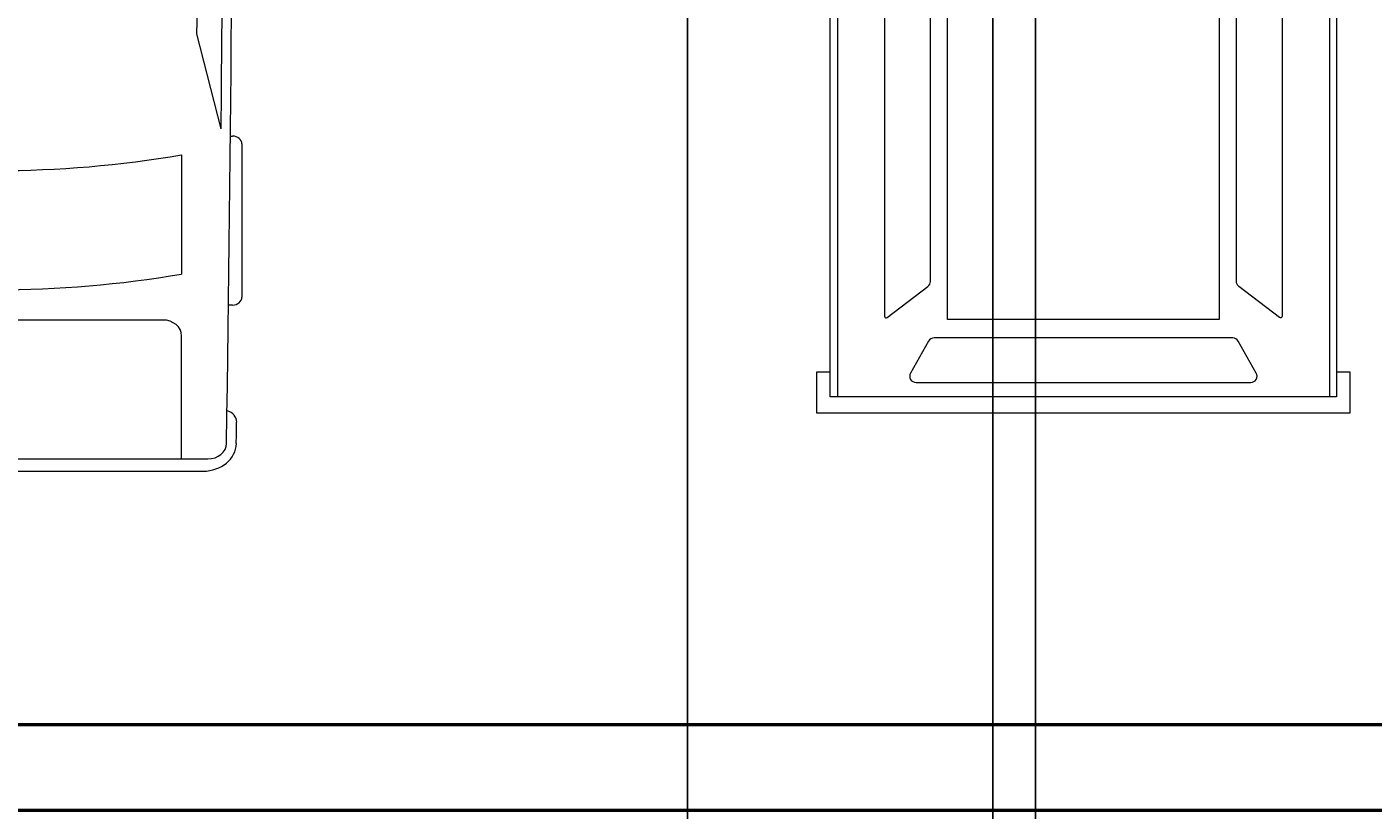
# Model space of a CAD drawing. Units: inches. Extents: x 5375 to 6084, y 16106 to 17259.
# Tile 10 of 32: x 5844 to 5986, y 16212 to 16295. Entities that reach past the tile are written whole.
import ezdxf

# ---------------------------------------------------------------- set-up
doc = ezdxf.new("R2010")
doc.units = ezdxf.units.IN
for name, color, linetype, lineweight in [('A-ANNO-DIMS', 2, 'Continuous', 18), ('C-PKNG-VEHI', 7, 'Continuous', 13), ('WALL', 6, 'Continuous', 50)]:
    doc.layers.add(name, color=color, linetype=linetype, lineweight=lineweight)
doc.styles.get("Standard").update_dxf_attribs({"font": 'arial.ttf'})
doc.dimstyles.get("Standard").update_dxf_attribs({"dimtxt": 0.18, "dimasz": 0.18, "dimexe": 0.18, "dimexo": 0.0625, "dimgap": 0.09, "dimtad": 0, "dimtih": 1, "dimtoh": 1, "dimdec": 4, "dimzin": 0, "dimdsep": 46, "dimtxsty": 'Standard', "dimcen": 0.09, "dimadec": 0, "dimazin": 0, "dimtfac": 1, "dimtdec": 4, "dimtofl": 0, "dimtmove": 0, "dimatfit": 3, "dimfxl": 1, "dimtolj": 1, "dimtzin": 0, "dimarcsym": 0})

# ---------------------------------------------------------------- blocks, each defined once
blk = doc.blocks.new('*U9')
for p, q in [((136.7, 38.89), (160.9, 38.89)), ((135.45, 37.07), (135.45, 37.41)), ((162.15, 37.41), (162.15, 36.77)), ((134.31, 35.6), (119.29, 31.78)), ((186.47, -33.5), (186.47, 33.5)), ((188.4, -32.76), (188.4, 32.76)), ((138.42, 29.35), (157.25, 29.35)), ((186.47, 29.35), (167.01, 29.35)), ((164.52, 26.39), (164.52, -26.39)), ((186.47, -10.53), (186.47, 10.53))]:
    blk.add_line(p, q)
for centre, major_axis, start_param, end_param in [((136.7, 37.41), (0, -1.48), 3.141593, 4.712389), ((160.9, 37.41), (0, 1.48), -1.570796, 0), ((64.48, -10555.62), (0, 10593.03), -0.013397, 0.002797), ((180.63, 35.84), (0, 2.22), -0.013017, 1.249894), ((64.48, -10556.36), (0, 10595.31), -0.013397, -0.013017), ((183.98, 33.5), (0, -2.96), 1.570796, 3.128196), ((183.98, 32.76), (0, -5.25), 1.570796, 3.128196), ((64.48, -10555.62), (0, -10591.55), 3.133765, 3.140441), ((95.79, -3666.35), (0, -3698.24), 3.134049, 3.144098), ((17.08, 0), (0, 147.02), 4.511394, 4.913384), ((35.91, 0), (0, 147.02), 4.511394, 4.913384), ((167.01, 26.39), (0, 2.96), 0, 1.570796)]:
    blk.add_ellipse(centre, major_axis=major_axis, ratio=0.842304, start_param=start_param, end_param=end_param)
blk = doc.blocks.new('*U10')
for p, q in [((1.28, 38.87), (175.66, 38.87)), ((1.28, -38.87), (175.66, -38.87))]:
    blk.add_line(p, q)
for points in [[(171.74, 40.01), (175.66, 40.01), (175.66, -40.01), (171.74, -40.01), (171.74, -42.18), (178.14, -42.18), (178.14, 42.18), (171.74, 42.18)], [(1.28, 40.01), (175.66, 40.01), (175.66, -40.01), (1.28, -40.01)], [(71.47, 21.48), (163.42, 21.48), (163.42, -21.48), (71.47, -21.48)]]:
    blk.add_lwpolyline(points, close=True)
for points in [[(102.19, 24.58), (106.97, 31, -0.236929), (107.78, 31.41), (162.91, 31.41, -0.621576), (163.11, 31), (158.19, 24.58, -0.233368), (157.39, 24.18), (102.39, 24.18, -0.616908)], [(171.88, 27.31), (166.83, 24.47, 0.271143), (166.32, 23.6), (166.32, -23.6, 0.271143), (166.83, -24.47), (171.88, -27.31, 0.573387), (173.37, -26.44), (173.37, 26.44, 0.573387)], [(102.19, -24.58), (106.97, -31, 0.236929), (107.78, -31.41), (162.91, -31.41, 0.621576), (163.11, -31), (158.19, -24.58, 0.233368), (157.39, -24.18), (102.39, -24.18, 0.616908)]]:
    blk.add_lwpolyline(points, format="xyb", close=True)
blk = doc.blocks.new('*D44')
at = {"layer": 'A-ANNO-DIMS', "color": 0, "lineweight": -2, "transparency": 16777216}
for p, q in [((5914, 16886.53), (5914, 16106.48)), ((5946.12, 16886.53), (5946.12, 16106.48)), ((5914.18, 16106.66), (5929.6, 16106.66)), ((5945.94, 16106.66), (5930.53, 16106.66))]:
    blk.add_line(p, q, dxfattribs=at)
at = {"layer": 'A-ANNO-DIMS', "color": 0, "transparency": 16777216}
for points in [[(5914.18, 16106.69), (5914.18, 16106.63), (5914, 16106.66)], [(5945.94, 16106.69), (5945.94, 16106.63), (5946.12, 16106.66)]]:
    blk.add_solid(points, dxfattribs=at)
at = {"layer": 'Defpoints', "color": 0, "transparency": 16777216}
for p in [(5914, 16886.6), (5946.12, 16886.6), (5914, 16106.66)]:
    blk.add_point(p, dxfattribs=at)
at = {"layer": 'A-ANNO-DIMS', "color": 0, "transparency": 16777216, "insert": (5930.06, 16106.66), "char_height": 0.18, "attachment_point": 5}
blk.add_mtext('\\A1;32.117', dxfattribs=at)
blk = doc.blocks.new('*D46')
at = {"layer": 'A-ANNO-DIMS', "color": 0, "lineweight": -2, "transparency": 16777216}
for p, q in [((5946.12, 16771.52), (5946.12, 16106.48)), ((5950.62, 16771.52), (5950.62, 16106.48)), ((5946.3, 16106.66), (5948.11, 16106.66)), ((5950.44, 16106.66), (5948.63, 16106.66))]:
    blk.add_line(p, q, dxfattribs=at)
at = {"layer": 'A-ANNO-DIMS', "color": 0, "transparency": 16777216}
for points in [[(5946.3, 16106.69), (5946.3, 16106.63), (5946.12, 16106.66)], [(5950.44, 16106.69), (5950.44, 16106.63), (5950.62, 16106.66)]]:
    blk.add_solid(points, dxfattribs=at)
at = {"layer": 'Defpoints', "color": 0, "transparency": 16777216}
for p in [(5946.12, 16771.58), (5950.62, 16771.58), (5950.62, 16106.66)]:
    blk.add_point(p, dxfattribs=at)
at = {"layer": 'A-ANNO-DIMS', "color": 0, "transparency": 16777216, "insert": (5948.37, 16106.66), "char_height": 0.18, "attachment_point": 5}
blk.add_mtext('\\A1;4.5', dxfattribs=at)

msp = doc.modelspace()

# ---------------------------------------------------------------- linework, layer by layer
at = {"layer": 'WALL'}
for p, q in [((5479.6199, 16221.3785), (6022.6199, 16221.3785)), ((5470.6199, 16212.3785), (6031.6199, 16212.3785))]:
    msp.add_line(p, q, dxfattribs=at)

# ---------------------------------------------------------------- block references
at = {"layer": 'C-PKNG-VEHI', "xscale": 0.6659567702331713, "yscale": 0.6659567702331713, "zscale": 0.6659567702331713, "rotation": 270}
for name, p in [('*U9', (5841.1969, 16373.5119)), ('*U10', (5955.6438, 16372.8314))]:
    msp.add_blockref(name, p, dxfattribs=at)

# ---------------------------------------------------------------- dimensions: what is measured, and where the dimension line sits
at = {"layer": 'A-ANNO-DIMS'}
for base, p1, p2, override, picture, middle in [((5914.0033, 16106.6631), (5946.1199, 16886.5956), (5914.0033, 16886.5956), {"dimdec": 3, "dimlfac": 1, "dimrnd": 0, "dimzin": 0, "dimdsep": 46, "dimlunit": 2}, '*D44', (5930.0616, 16106.6631)), ((5950.6199, 16106.6631), (5946.1199, 16771.5793), (5950.6199, 16771.5793), {"dimdec": 1, "dimlfac": 1, "dimrnd": 0, "dimzin": 0, "dimdsep": 46, "dimlunit": 2}, '*D46', (5948.3699, 16106.6631))]:
    dim = msp.add_linear_dim(base=base, p1=p1, p2=p2, dimstyle='Standard', override=override, dxfattribs=at)
    dim.commit()
    dim.dimension.update_dxf_attribs({"geometry": picture, "text_midpoint": middle})

doc.saveas('drawing.dxf')
